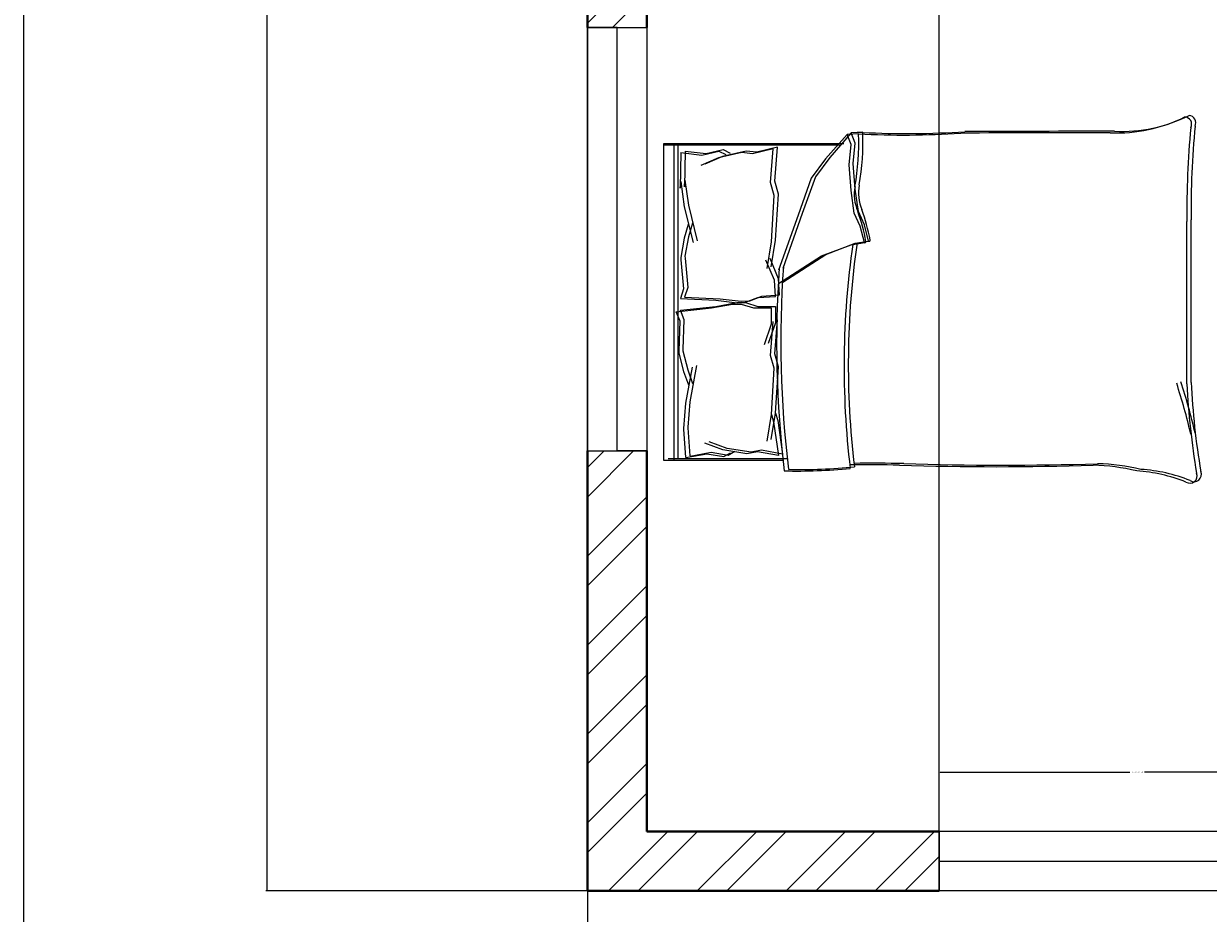
# Model space of a CAD drawing. Units: inches. Extents: x 1601 to 2297, y 1496 to 2631.
# Tile 2 of 57: x 1601 to 1780, y 1632 to 1767. Entities that reach past the tile are written whole.
import ezdxf

# ---------------------------------------------------------------- set-up
doc = ezdxf.new("R2010")
doc.units = ezdxf.units.IN
for name, color, linetype, lineweight in [('A-ANNO-DIMS', 2, 'Continuous', 18), ('A-ANNO-TTLB', 7, 'Continuous', 25), ('A-FURN', 8, 'Continuous', 18), ('A-GLAZ', 161, 'Continuous', 20), ('A-WALL', 7, 'Continuous', 40), ('A-WALL-PATT', 215, 'Continuous', 13)]:
    doc.layers.add(name, color=color, linetype=linetype, lineweight=lineweight)
doc.styles.get("Standard").update_dxf_attribs({"font": 'arial.ttf'})
doc.dimstyles.get("Standard").update_dxf_attribs({"dimtxt": 0.18, "dimasz": 0.18, "dimexe": 0.18, "dimexo": 0.0625, "dimgap": 0.09, "dimtad": 0, "dimtih": 1, "dimtoh": 1, "dimdec": 4, "dimzin": 0, "dimdsep": 46, "dimtxsty": 'Standard', "dimcen": 0.09, "dimadec": 0, "dimazin": 0, "dimtfac": 1, "dimtdec": 4, "dimtofl": 0, "dimtmove": 0, "dimatfit": 3, "dimfxl": 1, "dimtolj": 1, "dimtzin": 0, "dimarcsym": 0})

# ---------------------------------------------------------------- blocks, each defined once
blk = doc.blocks.new('BED-DOUBLE')
for p, q in [((27.75, 52.87), (24.5, 49.16)), ((27.75, 52.87), (24.5, 49.16)), ((27.75, 52.87), (24.5, 49.16)), ((27.75, 52.87), (24.5, 49.16)), ((28.39, 53.1), (25.13, 49.39)), ((28.39, 53.1), (25.13, 49.39)), ((28.39, 53.1), (25.13, 49.39)), ((28.39, 53.1), (25.13, 49.39)), ((29.49, 52.95), (27.75, 52.87, 3.87)), ((29.49, 52.95), (27.75, 52.87, 3.87)), ((29.49, 52.95), (27.75, 52.87, 3.87)), ((29.49, 52.95), (27.75, 52.87, 3.87)), ((28.36, 51.33), (27.75, 52.87)), ((28.36, 51.33), (27.75, 52.87)), ((28.36, 51.33), (27.75, 52.87)), ((28.36, 51.33), (27.75, 52.87)), ((30.13, 53.18), (28.39, 53.1, 3.87)), ((30.13, 53.18), (28.39, 53.1, 3.87)), ((30.13, 53.17), (28.39, 53.1, 3.87)), ((30.13, 53.17), (28.39, 53.1, 3.87)), ((29, 51.56), (28.39, 53.1)), ((29, 51.56), (28.39, 53.1)), ((29, 51.56), (28.39, 53.1)), ((29, 51.56), (28.39, 53.1)), ((0, 51.49), (0.64, 51.49)), ((0, 3.47), (0, 51.49)), ((0, 51.49), (0.64, 51.49)), ((0, 3.47), (0, 51.49)), ((0, 51.27), (26.61, 51.27)), ((0, 51.27), (26.61, 51.27)), ((0, 51.26), (26.61, 51.26)), ((0, 51.26), (26.61, 51.26)), ((0.64, 51.49), (27.25, 51.49)), ((0.64, 51.49), (27.25, 51.49)), ((0.64, 51.49), (27.25, 51.49)), ((0.64, 51.49), (27.25, 51.49)), ((1.53, 3.47), (1.53, 51.27)), ((1.53, 3.47), (1.53, 51.27)), ((1.53, 3.47), (1.53, 51.26)), ((1.53, 3.47), (1.53, 51.26)), ((2.17, 3.7), (2.17, 51.49)), ((2.17, 3.7), (2.17, 51.49)), ((2.17, 3.7), (2.17, 51.49)), ((2.17, 3.7), (2.17, 51.49)), ((3.2, 50.34), (3.1, 44.94)), ((3.2, 50.34), (3.1, 44.94)), ((3.2, 50.34), (3.1, 44.94)), ((3.2, 50.34), (3.1, 44.94)), ((3.2, 50.34), (6.41, 49.96)), ((3.2, 50.34), (6.41, 49.96)), ((3.2, 50.34), (6.41, 49.96)), ((3.2, 50.34), (6.41, 49.96)), ((5.77, 49.73), (8.34, 50.33)), ((5.77, 49.73), (8.34, 50.33)), ((5.77, 49.73), (8.34, 50.33)), ((5.77, 49.73), (8.34, 50.33)), ((6.41, 49.96), (8.98, 50.56)), ((6.41, 49.96), (8.98, 50.56)), ((6.41, 49.96), (8.98, 50.56)), ((6.41, 49.96), (8.98, 50.56)), ((8.34, 50.33), (9.38, 49.81)), ((8.34, 50.33), (9.38, 49.81)), ((8.34, 50.33), (9.38, 49.81)), ((8.34, 50.33), (9.38, 49.81)), ((12.47, 50.34), (8.9, 49.54)), ((12.47, 50.34), (8.9, 49.54)), ((12.47, 50.34), (8.9, 49.54)), ((12.47, 50.34), (8.9, 49.54)), ((8.98, 50.56), (10.02, 50.04)), ((8.98, 50.56), (10.02, 50.04)), ((8.98, 50.56), (10.02, 50.04)), ((8.98, 50.56), (10.02, 50.04)), ((14.07, 50.15), (12.47, 50.34)), ((14.07, 50.15), (12.47, 50.34)), ((14.07, 50.15), (12.47, 50.34)), ((14.07, 50.15), (12.47, 50.34)), ((16.57, 50.7), (13.43, 49.92)), ((16.57, 50.7), (13.43, 49.92)), ((16.57, 50.7), (13.43, 49.92)), ((16.57, 50.7), (13.43, 49.92)), ((17.21, 50.93), (14.07, 50.15)), ((17.21, 50.93), (14.07, 50.15)), ((17.21, 50.93), (14.07, 50.15)), ((17.21, 50.93), (14.07, 50.15)), ((16.17, 45.57), (16.57, 50.7)), ((16.17, 45.57), (16.57, 50.7)), ((16.17, 45.57), (16.57, 50.7)), ((16.17, 45.57), (16.57, 50.7)), ((16.81, 45.79), (17.21, 50.93)), ((16.81, 45.79), (17.21, 50.93)), ((16.81, 45.79), (17.21, 50.93)), ((16.81, 45.79), (17.21, 50.93)), ((28.06, 48.23), (28.36, 51.33)), ((28.06, 48.23), (28.36, 51.33)), ((28.06, 48.23), (28.36, 51.33)), ((28.06, 48.23), (28.36, 51.33)), ((28.69, 48.46), (29, 51.56)), ((28.69, 48.46), (29, 51.56)), ((28.69, 48.46), (29, 51.56)), ((28.69, 48.46), (29, 51.56)), ((2.56, 50.11), (2.46, 44.71)), ((2.56, 50.11), (2.46, 44.71)), ((2.56, 50.11), (2.46, 44.71)), ((2.56, 50.11), (2.46, 44.71)), ((2.56, 50.11), (5.77, 49.73)), ((2.56, 50.11), (5.77, 49.73)), ((2.56, 50.11), (5.77, 49.73)), ((2.56, 50.11), (5.77, 49.73)), ((8.26, 49.31), (5.58, 48.13)), ((8.26, 49.31), (5.58, 48.13)), ((8.26, 49.31), (5.58, 48.13)), ((8.26, 49.31), (5.58, 48.13)), ((8.9, 49.54), (6.22, 48.36)), ((8.9, 49.54), (6.22, 48.36)), ((8.9, 49.54), (6.22, 48.36)), ((8.9, 49.54), (6.22, 48.36)), ((11.83, 50.11), (8.26, 49.31)), ((11.83, 50.11), (8.26, 49.31)), ((11.83, 50.11), (8.26, 49.31)), ((11.83, 50.11), (8.26, 49.31)), ((13.43, 49.92), (11.83, 50.11)), ((13.43, 49.92), (11.83, 50.11)), ((13.43, 49.92), (11.83, 50.11)), ((13.43, 49.92), (11.83, 50.11)), ((24.5, 49.16), (22.33, 46.22)), ((24.5, 49.16), (22.33, 46.22)), ((24.5, 49.16), (22.33, 46.22)), ((24.5, 49.16), (22.33, 46.22)), ((25.13, 49.39), (22.97, 46.45)), ((25.13, 49.39), (22.97, 46.45)), ((25.13, 49.39), (22.97, 46.45)), ((25.13, 49.39), (22.97, 46.45)), ((28.36, 44.36), (28.06, 48.23)), ((28.36, 44.36), (28.06, 48.23)), ((28.36, 44.36), (28.06, 48.23)), ((28.36, 44.36), (28.06, 48.23)), ((29, 44.59), (28.69, 48.46)), ((29, 44.59), (28.69, 48.46)), ((29, 44.59), (28.69, 48.46)), ((29, 44.59), (28.69, 48.46)), ((2.46, 44.71), (2.54, 45.71)), ((2.46, 44.71), (2.54, 45.71)), ((2.46, 44.71), (2.54, 45.71)), ((2.46, 44.71), (2.54, 45.71)), ((2.54, 45.71), (3.07, 41.91)), ((2.54, 45.71), (3.07, 41.91)), ((2.54, 45.71), (3.07, 41.91)), ((2.54, 45.71), (3.07, 41.91)), ((3.1, 44.94), (3.18, 45.94)), ((3.1, 44.94), (3.18, 45.94)), ((3.1, 44.94), (3.18, 45.94)), ((3.1, 44.94), (3.18, 45.94)), ((3.18, 45.94), (3.71, 42.14)), ((3.18, 45.94), (3.71, 42.14)), ((3.18, 45.94), (3.71, 42.14)), ((3.18, 45.94), (3.71, 42.14)), ((16.73, 43.61), (16.17, 45.57)), ((16.73, 43.61), (16.17, 45.57)), ((16.73, 43.61), (16.17, 45.57)), ((16.73, 43.61), (16.17, 45.57)), ((17.37, 43.83), (16.81, 45.79)), ((17.37, 43.83), (16.81, 45.79)), ((17.37, 43.83), (16.81, 45.79)), ((17.37, 43.83), (16.81, 45.79)), ((22.33, 46.22), (20.32, 40.64)), ((22.33, 46.22), (20.32, 40.64)), ((22.33, 46.22), (20.32, 40.64)), ((22.33, 46.22), (20.32, 40.64)), ((22.97, 46.45), (20.96, 40.87)), ((22.97, 46.45), (20.96, 40.87)), ((22.97, 46.45), (20.96, 40.87)), ((22.97, 46.45), (20.96, 40.87)), ((16.3, 36.6), (16.73, 43.61)), ((16.3, 36.6), (16.73, 43.61)), ((16.3, 36.6), (16.73, 43.61)), ((16.3, 36.6), (16.73, 43.61)), ((16.93, 36.82), (17.37, 43.83)), ((16.93, 36.82), (17.37, 43.83)), ((16.93, 36.82), (17.37, 43.83)), ((16.93, 36.82), (17.37, 43.83)), ((28.83, 40.95), (28.36, 44.36)), ((28.83, 40.95), (28.36, 44.36)), ((28.83, 40.95), (28.36, 44.36)), ((28.83, 40.95), (28.36, 44.36)), ((29.47, 41.18), (29, 44.59)), ((29.47, 41.18), (29, 44.59)), ((29.47, 41.18), (29, 44.59)), ((29.47, 41.18), (29, 44.59)), ((3.07, 41.91), (4.42, 36.49)), ((3.07, 41.91), (4.42, 36.49)), ((3.07, 41.91), (4.42, 36.49)), ((3.07, 41.91), (4.42, 36.49)), ((3.71, 42.14), (5.06, 36.72)), ((3.71, 42.14), (5.06, 36.72)), ((3.71, 42.14), (5.06, 36.72)), ((3.71, 42.14), (5.06, 36.72)), ((20.32, 40.64), (17.38, 32.31)), ((20.32, 40.64), (17.38, 32.31)), ((20.32, 40.64), (17.38, 32.31)), ((20.32, 40.64), (17.38, 32.31)), ((20.96, 40.87), (18.02, 32.53)), ((20.96, 40.87), (18.02, 32.53)), ((20.96, 40.87), (18.02, 32.53)), ((20.96, 40.87), (18.02, 32.53)), ((29.76, 38.94), (28.83, 40.95)), ((29.76, 38.94), (28.83, 40.95)), ((29.76, 38.94), (28.83, 40.95)), ((29.76, 38.94), (28.83, 40.95)), ((30.4, 39.17), (29.47, 41.18)), ((30.4, 39.17), (29.47, 41.18)), ((30.4, 39.17), (29.47, 41.18)), ((30.4, 39.17), (29.47, 41.18)), ((79.24, 15.06), (79.24, 39.68)), ((79.24, 15.06), (79.24, 39.68)), ((79.24, 15.06), (79.24, 39.68)), ((79.24, 15.06), (79.24, 39.68)), ((79.88, 15.29), (79.88, 39.91)), ((79.88, 15.29), (79.88, 39.91)), ((79.88, 15.29), (79.88, 39.91)), ((79.88, 15.29), (79.88, 39.91)), ((3.67, 39.2), (3.08, 37.14)), ((3.67, 39.2), (3.08, 37.13)), ((3.67, 39.2), (3.08, 37.14)), ((3.67, 39.2), (3.08, 37.13)), ((4.31, 39.43), (3.72, 37.36)), ((4.31, 39.43), (3.72, 37.36)), ((4.31, 39.43), (3.72, 37.36)), ((4.31, 39.43), (3.72, 37.36)), ((30.38, 36.46), (29.76, 38.94)), ((30.38, 36.46), (29.76, 38.94)), ((30.38, 36.46), (29.76, 38.94)), ((30.38, 36.46), (29.76, 38.94)), ((31.02, 36.69), (30.4, 39.17)), ((31.02, 36.69), (30.4, 39.17)), ((31.02, 36.69), (30.4, 39.17)), ((31.02, 36.69), (30.4, 39.17)), ((3.08, 37.14), (2.54, 34.2)), ((3.08, 37.14), (2.54, 34.2)), ((3.08, 37.13), (2.54, 34.2)), ((3.08, 37.13), (2.54, 34.2)), ((3.72, 37.36), (3.18, 34.43)), ((3.72, 37.36), (3.18, 34.43)), ((3.72, 37.36), (3.18, 34.43)), ((3.72, 37.36), (3.18, 34.43)), ((15.63, 32.56), (16.3, 36.6)), ((15.63, 32.56), (16.3, 36.6)), ((15.63, 32.56), (16.3, 36.6)), ((15.63, 32.56), (16.3, 36.6)), ((16.27, 32.79), (16.93, 36.82)), ((16.27, 32.79), (16.93, 36.82)), ((16.27, 32.79), (16.93, 36.82)), ((16.27, 32.79), (16.93, 36.82)), ((23.88, 34.45), (28.36, 36.15)), ((23.88, 34.45), (28.36, 36.15)), ((23.88, 34.45), (28.36, 36.15)), ((23.88, 34.45), (28.36, 36.15)), ((24.52, 34.68), (29, 36.38)), ((24.52, 34.68), (29, 36.38)), ((24.52, 34.68), (29, 36.38)), ((24.52, 34.68), (29, 36.38)), ((28.36, 36.15), (30.38, 36.46)), ((28.36, 36.15), (30.38, 36.46)), ((28.36, 36.15), (30.38, 36.46)), ((28.36, 36.15), (30.38, 36.46)), ((29, 36.38), (31.02, 36.69)), ((29, 36.38), (31.02, 36.69)), ((29, 36.38), (31.02, 36.69)), ((29, 36.38), (31.02, 36.69)), ((2.54, 34.2), (2.56, 33.88)), ((2.54, 34.2), (2.56, 33.88)), ((2.54, 34.2), (2.56, 33.88)), ((2.54, 34.2), (2.56, 33.88)), ((3.18, 34.43), (3.2, 34.11)), ((3.18, 34.43), (3.2, 34.11)), ((3.18, 34.43), (3.2, 34.11)), ((3.18, 34.43), (3.2, 34.11)), ((3.2, 34.11), (3.62, 29.68)), ((3.2, 34.11), (3.62, 29.68)), ((3.2, 34.11), (3.62, 29.68)), ((3.2, 34.11), (3.62, 29.68)), ((17.38, 30.26), (23.88, 34.45)), ((17.38, 30.26), (23.88, 34.45)), ((17.38, 30.26), (23.88, 34.45)), ((17.38, 30.26), (23.88, 34.45)), ((18.02, 30.49), (24.52, 34.68)), ((18.02, 30.49), (24.52, 34.68)), ((18.02, 30.49), (24.52, 34.68)), ((18.02, 30.49), (24.52, 34.68)), ((2.56, 33.88), (2.98, 29.46)), ((2.56, 33.88), (2.98, 29.46)), ((2.56, 33.88), (2.98, 29.46)), ((2.56, 33.88), (2.98, 29.46)), ((16.74, 30.75), (15.45, 33.82)), ((16.74, 30.75), (15.45, 33.82)), ((16.74, 30.75), (15.45, 33.82)), ((16.74, 30.75), (15.45, 33.82)), ((17.38, 30.98), (16.09, 34.05)), ((17.38, 30.98), (16.09, 34.05)), ((17.38, 30.98), (16.09, 34.05)), ((17.38, 30.98), (16.09, 34.05)), ((16.89, 28.3), (16.74, 30.75)), ((16.89, 28.3), (16.74, 30.75)), ((16.89, 28.3), (16.74, 30.75)), ((16.89, 28.3), (16.74, 30.75)), ((17.53, 28.53), (17.38, 30.98)), ((17.53, 28.53), (17.38, 30.98)), ((17.53, 28.53), (17.38, 30.98)), ((17.53, 28.53), (17.38, 30.98)), ((2.98, 29.46), (2.49, 27.98)), ((2.98, 29.46), (2.49, 27.98)), ((2.98, 29.46), (2.49, 27.98)), ((2.98, 29.46), (2.49, 27.98)), ((3.62, 29.68), (3.13, 28.21)), ((3.62, 29.68), (3.13, 28.2)), ((3.62, 29.68), (3.13, 28.21)), ((3.62, 29.68), (3.13, 28.2)), ((2.49, 27.98), (7.87, 27.73)), ((2.49, 27.98), (7.87, 27.73)), ((2.49, 27.98), (7.87, 27.73)), ((2.49, 27.98), (7.87, 27.73)), ((3.13, 28.21), (8.51, 27.96)), ((3.13, 28.21), (8.51, 27.96)), ((3.13, 28.2), (8.51, 27.96)), ((3.13, 28.2), (8.51, 27.96)), ((7.22, 26.56), (10.4, 27.14)), ((7.22, 26.56), (10.4, 27.14)), ((7.22, 26.56), (10.4, 27.14)), ((7.22, 26.56), (10.4, 27.14)), ((7.86, 26.79), (11.04, 27.37)), ((7.86, 26.79), (11.04, 27.37)), ((7.86, 26.79), (11.04, 27.37)), ((7.86, 26.79), (11.04, 27.37)), ((7.87, 27.73), (11.08, 27.35)), ((7.87, 27.73), (11.08, 27.35)), ((7.87, 27.73), (11.08, 27.35)), ((7.87, 27.73), (11.08, 27.35)), ((8.51, 27.96), (11.72, 27.58)), ((8.51, 27.96), (11.72, 27.58)), ((8.51, 27.96), (11.72, 27.58)), ((8.51, 27.96), (11.72, 27.58)), ((10.4, 27.14), (11.7, 27.14)), ((10.4, 27.14), (11.7, 27.14)), ((10.4, 27.14), (11.7, 27.14)), ((10.4, 27.14), (11.7, 27.14)), ((11.04, 27.37), (12.34, 27.37)), ((11.04, 27.37), (12.34, 27.37)), ((11.04, 27.37), (12.34, 27.37)), ((11.04, 27.37), (12.34, 27.37)), ((11.08, 27.35), (12.38, 27.44)), ((11.08, 27.35), (12.38, 27.44)), ((11.08, 27.35), (12.38, 27.44)), ((11.08, 27.35), (12.38, 27.44)), ((11.7, 27.14), (13.58, 26.56)), ((11.7, 27.14), (13.58, 26.56)), ((11.7, 27.14), (13.58, 26.56)), ((11.7, 27.14), (13.58, 26.56)), ((11.72, 27.58), (13.02, 27.66)), ((11.72, 27.58), (13.02, 27.66)), ((11.72, 27.58), (13.02, 27.66)), ((11.72, 27.58), (13.02, 27.66)), ((12.34, 27.37), (14.22, 26.79)), ((12.34, 27.37), (14.22, 26.79)), ((12.34, 27.37), (14.22, 26.79)), ((12.34, 27.37), (14.22, 26.79)), ((12.38, 27.44), (14.22, 28.13)), ((12.38, 27.44), (14.22, 28.13)), ((12.38, 27.44), (14.22, 28.13)), ((12.38, 27.44), (14.22, 28.13)), ((13.02, 27.66), (14.86, 28.36)), ((13.02, 27.66), (14.86, 28.36)), ((13.02, 27.66), (14.86, 28.36)), ((13.02, 27.66), (14.86, 28.36)), ((14.22, 28.13), (16.89, 28.3)), ((14.22, 28.13), (16.89, 28.3)), ((14.22, 28.13), (16.89, 28.3)), ((14.22, 28.13), (16.89, 28.3)), ((14.86, 28.36), (17.53, 28.53)), ((14.86, 28.36), (17.53, 28.53)), ((14.86, 28.36), (17.53, 28.53)), ((14.86, 28.36), (17.53, 28.53)), ((1.87, 25.98), (7.22, 26.56)), ((1.87, 25.98), (7.22, 26.56)), ((1.87, 25.98), (7.22, 26.56)), ((1.87, 25.98), (7.22, 26.56)), ((2.45, 24.54), (1.87, 25.98)), ((2.45, 24.54), (1.87, 25.98)), ((2.45, 24.54), (1.87, 25.98)), ((2.45, 24.54), (1.87, 25.98)), ((2.51, 26.21), (7.86, 26.79)), ((2.51, 26.21), (7.86, 26.79)), ((2.51, 26.21), (7.86, 26.79)), ((2.51, 26.21), (7.86, 26.79)), ((3.09, 24.77), (2.51, 26.21)), ((3.09, 24.76), (2.51, 26.21)), ((3.09, 24.77), (2.51, 26.21)), ((3.09, 24.76), (2.51, 26.21)), ((13.58, 26.56), (16.26, 26.56)), ((13.58, 26.56), (16.26, 26.56)), ((13.58, 26.56), (16.26, 26.56)), ((13.58, 26.56), (16.26, 26.56)), ((14.22, 26.79), (16.9, 26.79)), ((14.22, 26.79), (16.9, 26.79)), ((14.22, 26.79), (16.9, 26.79)), ((14.22, 26.79), (16.9, 26.79)), ((16.26, 26.56), (16.26, 24.1)), ((16.26, 26.56), (16.26, 24.1)), ((16.26, 26.56), (16.26, 24.1)), ((16.26, 26.56), (16.26, 24.1)), ((16.9, 26.79), (16.9, 24.33)), ((16.9, 26.79), (16.9, 24.33)), ((16.9, 26.79), (16.9, 24.33)), ((16.9, 26.79), (16.9, 24.33)), ((2.3, 20.09), (2.45, 24.54)), ((2.3, 20.09), (2.45, 24.54)), ((2.3, 20.09), (2.45, 24.54)), ((2.3, 20.09), (2.45, 24.54)), ((2.94, 20.32), (3.09, 24.77)), ((2.94, 20.32), (3.09, 24.77)), ((2.94, 20.32), (3.09, 24.76)), ((2.94, 20.32), (3.09, 24.76)), ((16.26, 24.1), (15.17, 20.96)), ((16.26, 24.1), (15.17, 20.96)), ((16.26, 24.1), (15.17, 20.96)), ((16.26, 24.1), (15.17, 20.96)), ((16.9, 24.33), (15.81, 21.19)), ((16.9, 24.33), (15.81, 21.19)), ((16.9, 24.33), (15.81, 21.19)), ((16.9, 24.33), (15.81, 21.19)), ((16.17, 19.38), (16.57, 24.52)), ((16.17, 19.38), (16.57, 24.52)), ((16.17, 19.38), (16.57, 24.52)), ((16.17, 19.38), (16.57, 24.52)), ((16.81, 19.61), (17.21, 24.74)), ((16.81, 19.61), (17.21, 24.74)), ((16.81, 19.61), (17.21, 24.74)), ((16.81, 19.61), (17.21, 24.74)), ((2.3, 19.77), (2.3, 20.09)), ((2.3, 19.77), (2.3, 20.09)), ((2.3, 19.77), (2.3, 20.09)), ((2.3, 19.77), (2.3, 20.09)), ((3.03, 16.88), (2.3, 19.77)), ((3.03, 16.88), (2.3, 19.77)), ((3.03, 16.88), (2.3, 19.77)), ((3.03, 16.88), (2.3, 19.77)), ((2.94, 20), (2.94, 20.32)), ((2.94, 20), (2.94, 20.32)), ((2.94, 20), (2.94, 20.32)), ((2.94, 20), (2.94, 20.32)), ((3.67, 17.11), (2.94, 20)), ((3.67, 17.11), (2.94, 20)), ((3.67, 17.11), (2.94, 20)), ((3.67, 17.11), (2.94, 20)), ((16.73, 17.42), (16.17, 19.38)), ((16.73, 17.42), (16.17, 19.38)), ((16.73, 17.42), (16.17, 19.38)), ((16.73, 17.42), (16.17, 19.38)), ((17.37, 17.65), (16.81, 19.61)), ((17.37, 17.65), (16.81, 19.61)), ((17.37, 17.65), (16.81, 19.61)), ((17.37, 17.65), (16.81, 19.61)), ((3.75, 14.85), (3.03, 16.88)), ((3.75, 14.85), (3.03, 16.88)), ((3.75, 14.85), (3.03, 16.88)), ((3.75, 14.85), (3.03, 16.88)), ((3.32, 12.11), (4.33, 17.6)), ((3.32, 12.11), (4.33, 17.6)), ((3.32, 12.11), (4.33, 17.6)), ((3.32, 12.11), (4.33, 17.6)), ((4.39, 15.08), (3.67, 17.11)), ((4.39, 15.08), (3.67, 17.11)), ((4.39, 15.08), (3.67, 17.11)), ((4.39, 15.08), (3.67, 17.11)), ((3.96, 12.34), (4.97, 17.83)), ((3.96, 12.34), (4.97, 17.83)), ((3.96, 12.34), (4.97, 17.83)), ((3.96, 12.34), (4.97, 17.83)), ((16.3, 10.41), (16.73, 17.42)), ((16.3, 10.41), (16.73, 17.42)), ((16.3, 10.41), (16.73, 17.42)), ((16.3, 10.41), (16.73, 17.42)), ((16.93, 10.64), (17.37, 17.65)), ((16.93, 10.64), (17.37, 17.65)), ((16.93, 10.64), (17.37, 17.65)), ((16.93, 10.64), (17.37, 17.65)), ((3.03, 8.28), (3.32, 12.11)), ((3.03, 8.28), (3.32, 12.11)), ((3.03, 8.28), (3.32, 12.11)), ((3.03, 8.28), (3.32, 12.11)), ((3.67, 8.51), (3.96, 12.34)), ((3.67, 8.51), (3.96, 12.34)), ((3.67, 8.51), (3.96, 12.34)), ((3.67, 8.51), (3.96, 12.34)), ((15.63, 6.38), (16.3, 10.41)), ((15.63, 6.38), (16.3, 10.41)), ((15.63, 6.38), (16.3, 10.41)), ((15.63, 6.38), (16.3, 10.41)), ((16.27, 6.61), (16.93, 10.64)), ((16.27, 6.61), (16.93, 10.64)), ((16.27, 6.61), (16.93, 10.64)), ((16.27, 6.61), (16.93, 10.64)), ((16.3, 10.41), (16.62, 9.28)), ((16.3, 10.41), (16.62, 9.28)), ((16.3, 10.41), (16.62, 9.28)), ((16.3, 10.41), (16.62, 9.28)), ((16.62, 9.28), (17.34, 4.18)), ((16.62, 9.28), (17.34, 4.18)), ((16.62, 9.28), (17.34, 4.18)), ((16.62, 9.28), (17.34, 4.18)), ((16.93, 10.64), (17.26, 9.51)), ((16.93, 10.64), (17.26, 9.51)), ((16.93, 10.64), (17.26, 9.51)), ((16.93, 10.64), (17.26, 9.51)), ((17.26, 9.51), (17.98, 4.41)), ((17.26, 9.51), (17.98, 4.41)), ((17.26, 9.51), (17.98, 4.41)), ((17.26, 9.51), (17.98, 4.41)), ((3.01, 8.18), (3.03, 8.28)), ((3.01, 8.18), (3.03, 8.28)), ((3.01, 8.18), (3.03, 8.28)), ((3.01, 8.18), (3.03, 8.28)), ((3.34, 3.9), (3.01, 8.18)), ((3.34, 3.9), (3.01, 8.18)), ((3.34, 3.9), (3.01, 8.18)), ((3.34, 3.9), (3.01, 8.18)), ((3.65, 8.41), (3.67, 8.51)), ((3.65, 8.41), (3.67, 8.51)), ((3.65, 8.41), (3.67, 8.51)), ((3.65, 8.41), (3.67, 8.51)), ((3.98, 4.13), (3.65, 8.41)), ((3.98, 4.13), (3.65, 8.41)), ((3.98, 4.13), (3.65, 8.41)), ((3.98, 4.13), (3.65, 8.41)), ((8.95, 5.05), (6.21, 6.06)), ((8.95, 5.05), (6.21, 6.06)), ((8.95, 5.05), (6.21, 6.06)), ((8.95, 5.05), (6.21, 6.06)), ((9.59, 5.28), (6.85, 6.29)), ((9.59, 5.28), (6.85, 6.29)), ((9.59, 5.28), (6.85, 6.29)), ((9.59, 5.28), (6.85, 6.29)), ((18.75, 3.7), (0.64, 3.7)), ((18.75, 3.7), (0.64, 3.7)), ((18.75, 3.7), (0.64, 3.7)), ((18.75, 3.7), (0.64, 3.7)), ((3.32, 3.89), (6.5, 4.47)), ((3.32, 3.89), (6.5, 4.47)), ((3.32, 3.89), (6.5, 4.47)), ((3.32, 3.89), (6.5, 4.47)), ((3.96, 4.12), (7.14, 4.7)), ((3.96, 4.12), (7.14, 4.7)), ((3.96, 4.12), (7.14, 4.7)), ((3.96, 4.12), (7.14, 4.7)), ((6.5, 4.47), (9.1, 4.04)), ((6.5, 4.47), (9.1, 4.04)), ((6.5, 4.47), (9.1, 4.04)), ((6.5, 4.47), (9.1, 4.04)), ((7.14, 4.7), (9.74, 4.27)), ((7.14, 4.7), (9.74, 4.27)), ((7.14, 4.7), (9.74, 4.27)), ((7.14, 4.7), (9.74, 4.27)), ((12.57, 4.47), (8.95, 5.05)), ((12.57, 4.47), (8.95, 5.05)), ((12.57, 4.47), (8.95, 5.05)), ((12.57, 4.47), (8.95, 5.05)), ((9.1, 4.04), (10.11, 4.62)), ((9.1, 4.04), (10.11, 4.62)), ((9.1, 4.04), (10.11, 4.62)), ((9.1, 4.04), (10.11, 4.62)), ((13.21, 4.7), (9.59, 5.28)), ((13.21, 4.7), (9.59, 5.28)), ((13.21, 4.7), (9.59, 5.28)), ((13.21, 4.7), (9.59, 5.28)), ((9.74, 4.27), (10.75, 4.85)), ((9.74, 4.27), (10.75, 4.85)), ((9.74, 4.27), (10.75, 4.85)), ((9.74, 4.27), (10.75, 4.85)), ((14.16, 4.76), (12.57, 4.47)), ((14.16, 4.76), (12.57, 4.47)), ((14.16, 4.76), (12.57, 4.47)), ((14.16, 4.76), (12.57, 4.47)), ((14.8, 4.99), (13.21, 4.7)), ((14.8, 4.99), (13.21, 4.7)), ((14.8, 4.99), (13.21, 4.7)), ((14.8, 4.99), (13.21, 4.7)), ((17.34, 4.18), (14.16, 4.76)), ((17.34, 4.18), (14.16, 4.76)), ((17.34, 4.18), (14.16, 4.76)), ((17.34, 4.18), (14.16, 4.76)), ((17.98, 4.41), (14.8, 4.99)), ((17.98, 4.41), (14.8, 4.99)), ((17.98, 4.41), (14.8, 4.99)), ((17.98, 4.41), (14.8, 4.99)), ((18.11, 3.47), (0, 3.47)), ((18.11, 3.47), (0, 3.47)), ((18.11, 3.47), (0, 3.47)), ((18.11, 3.47), (0, 3.47))]:
    blk.add_line(p, q)
for centre, radius, start, end in [((69.31, 76.39), 23.07, 267.4714, 296.4681), ((69.31, 76.39), 23.07, 267.4714, 296.4681), ((69.31, 76.39), 23.07, 267.4714, 296.4681), ((69.31, 76.39), 23.07, 267.4714, 296.4681), ((79.51, 54.64), 1.1, 332.6588, 86.02), ((79.51, 54.64), 1.1, 332.6588, 86.02), ((79.51, 54.64), 1.1, 332.6588, 86.02), ((79.51, 54.64), 1.1, 332.6588, 86.02), ((68.67, 76.16), 23.07, 267.4714, 296.4681), ((68.67, 76.16), 23.07, 267.4714, 296.4681), ((68.67, 76.16), 23.07, 267.4714, 296.4681), ((68.67, 76.16), 23.07, 267.4714, 296.4681), ((78.87, 54.41), 1.1, 332.6588, 86.02), ((78.87, 54.41), 1.1, 332.6588, 86.02), ((78.87, 54.41), 1.1, 332.6588, 86.02), ((78.87, 54.41), 1.1, 332.6588, 86.02), ((212.28, 41.15), 133.04, 174.4998, 180.6351), ((212.28, 41.15), 133.04, 174.4998, 180.6351), ((212.28, 41.15), 133.04, 174.4998, 180.6351), ((212.28, 41.15), 133.04, 174.4998, 180.6351), ((212.92, 41.38), 133.04, 174.4998, 180.6351), ((212.92, 41.38), 133.04, 174.4998, 180.6351), ((212.92, 41.38), 133.04, 174.4998, 180.6351), ((212.92, 41.38), 133.04, 174.4998, 180.6351), ((-6.66, 51.33), 36.18, 349.8763, 2.5657), ((-6.66, 51.33), 36.18, 349.8763, 2.5657), ((-6.66, 51.33), 36.18, 349.8763, 2.5657), ((-6.66, 51.33), 36.18, 349.8763, 2.5657), ((36.31, 182.27), 129.5, 266.9791, 273.8365), ((36.31, 182.27), 129.5, 266.9791, 273.8365), ((36.31, 182.27), 129.5, 266.9791, 273.8365), ((36.31, 182.27), 129.5, 266.9791, 273.8365), ((-6.02, 51.56), 36.18, 349.8763, 2.5657), ((-6.02, 51.56), 36.18, 349.8763, 2.5657), ((-6.02, 51.56), 36.18, 349.8763, 2.5657), ((-6.02, 51.56), 36.18, 349.8763, 2.5657), ((36.95, 182.49), 129.5, 266.9791, 273.8365), ((36.95, 182.49), 129.5, 266.9791, 273.8365), ((36.95, 182.49), 129.5, 266.9791, 273.8365), ((36.95, 182.49), 129.5, 266.9791, 273.8365), ((67.82, -4508.74), 4561.86, 90.00217, 90.28689), ((67.82, -4508.74), 4561.86, 90.00217, 90.28689), ((67.82, -4508.74), 4561.86, 90.00217, 90.28689), ((67.82, -4508.74), 4561.86, 90.00217, 90.28689), ((68.46, -4508.52), 4561.86, 90.00217, 90.28689), ((68.46, -4508.52), 4561.86, 90.00217, 90.28689), ((68.46, -4508.52), 4561.86, 90.00217, 90.28689), ((68.46, -4508.52), 4561.86, 90.00217, 90.28689), ((35.07, 43.74), 6.22, 168.6608, 203.7384), ((35.07, 43.74), 6.22, 168.6608, 203.7384), ((35.07, 43.74), 6.22, 168.6608, 203.7384), ((35.07, 43.74), 6.22, 168.6608, 203.7384), ((35.71, 43.97), 6.22, 168.6608, 203.7384), ((35.71, 43.97), 6.22, 168.6608, 203.7384), ((35.71, 43.97), 6.22, 168.6608, 203.7384), ((35.71, 43.97), 6.22, 168.6608, 203.7384), ((2.12, 31.38), 29.65, 10.6617, 19.8806), ((2.12, 31.38), 29.65, 10.6617, 19.8806), ((2.12, 31.38), 29.65, 10.6617, 19.8806), ((2.12, 31.38), 29.65, 10.6617, 19.8806), ((1.48, 31.15), 29.65, 10.6617, 19.8806), ((1.48, 31.15), 29.65, 10.6617, 19.8806), ((1.48, 31.15), 29.65, 10.6617, 19.8806), ((1.48, 31.15), 29.65, 10.6617, 19.8806), ((156.32, 17.76), 129.02, 171.7845, 186.9006), ((156.32, 17.76), 129.02, 171.7845, 186.9006), ((156.32, 17.76), 129.02, 171.7845, 186.9006), ((156.32, 17.76), 129.02, 171.7845, 186.9006), ((156.96, 17.98), 129.02, 171.7845, 186.9006), ((156.96, 17.98), 129.02, 171.7845, 186.9006), ((156.96, 17.98), 129.02, 171.7845, 186.9006), ((156.96, 17.98), 129.02, 171.7845, 186.9006), ((30.44, 36.64), 0.185, 250.2464, 1.1377), ((30.44, 36.64), 0.185, 250.2464, 1.1377), ((30.44, 36.64), 0.185, 250.2464, 1.1377), ((30.44, 36.64), 0.185, 250.2464, 1.1377), ((31.08, 36.86), 0.185, 250.2464, 1.1377), ((31.08, 36.86), 0.185, 250.2464, 1.1377), ((31.08, 36.86), 0.185, 250.2464, 1.1377), ((31.08, 36.86), 0.185, 250.2464, 1.1377), ((182.05, 21.36), 164.97, 176.0865, 186.7821), ((182.05, 21.36), 164.97, 176.0865, 186.7821), ((182.05, 21.36), 164.97, 176.0865, 186.7821), ((182.05, 21.36), 164.97, 176.0865, 186.7821), ((182.69, 21.59), 164.97, 176.0865, 186.7821), ((182.69, 21.59), 164.97, 176.0865, 186.7821), ((182.69, 21.59), 164.97, 176.0865, 186.7821), ((182.69, 21.59), 164.97, 176.0865, 186.7821), ((-23.71, -17.22), 106.46, 13.3832, 17.7053), ((-23.71, -17.22), 106.46, 13.3832, 17.7053), ((-23.71, -17.22), 106.46, 13.3832, 17.7053), ((-23.71, -17.22), 106.46, 13.3832, 17.7053), ((-23.07, -16.99), 106.46, 13.3832, 17.7053), ((-23.07, -16.99), 106.46, 13.3832, 17.7053), ((-23.07, -16.99), 106.46, 13.3832, 17.7053), ((-23.07, -16.99), 106.46, 13.3832, 17.7053), ((200.84, 21.43), 121.76, 182.9958, 189.4091), ((200.84, 21.43), 121.76, 182.9958, 189.4091), ((200.84, 21.43), 121.76, 182.9958, 189.4091), ((200.84, 21.43), 121.76, 182.9958, 189.4091), ((201.48, 21.65), 121.76, 182.9958, 189.4091), ((201.48, 21.65), 121.76, 182.9958, 189.4091), ((201.48, 21.65), 121.76, 182.9958, 189.4091), ((201.48, 21.65), 121.76, 182.9958, 189.4091), ((20.1, 85.16), 83.31, 268.7218, 275.604), ((20.1, 85.16), 83.31, 268.7218, 275.604), ((20.1, 85.16), 83.31, 268.7218, 275.604), ((20.1, 85.16), 83.31, 268.7218, 275.604), ((20.74, 85.39), 83.31, 268.7218, 275.604), ((20.74, 85.39), 83.31, 268.7218, 275.604), ((20.74, 85.39), 83.31, 268.7218, 275.604), ((20.74, 85.39), 83.31, 268.7218, 275.604), ((31.17, -167.31), 170.11, 88.4762, 91.0082), ((31.17, -167.31), 170.11, 88.4762, 91.0082), ((31.17, -167.31), 170.11, 88.4762, 91.0082), ((31.17, -167.31), 170.11, 88.4762, 91.0082), ((31.81, -167.08), 170.11, 88.4762, 91.0082), ((31.81, -167.08), 170.11, 88.4762, 91.0082), ((31.81, -167.08), 170.11, 88.4762, 91.0082), ((31.81, -167.08), 170.11, 88.4762, 91.0082), ((50.61, 484.82), 482.31, 268.2277, 271.7185), ((50.61, 484.82), 482.31, 268.2277, 271.7185), ((50.61, 484.82), 482.31, 268.2277, 271.7185), ((50.61, 484.82), 482.31, 268.2277, 271.7185), ((51.25, 485.05), 482.31, 268.2277, 271.7185), ((51.25, 485.05), 482.31, 268.2277, 271.7185), ((51.25, 485.05), 482.31, 268.2277, 271.7185), ((51.25, 485.05), 482.31, 268.2277, 271.7185), ((64.51, -26.9), 29.63, 76.0648, 88.9113), ((64.51, -26.9), 29.63, 76.0648, 88.9113), ((64.51, -26.9), 29.63, 76.0648, 88.9113), ((64.51, -26.9), 29.63, 76.0648, 88.9113), ((65.15, -26.67), 29.63, 76.0648, 88.9113), ((65.15, -26.67), 29.63, 76.0648, 88.9113), ((65.15, -26.67), 29.63, 76.0648, 88.9113), ((65.15, -26.67), 29.63, 76.0648, 88.9113), ((70.28, -21.66), 23.56, 67.9751, 86.652), ((70.28, -21.66), 23.56, 67.9751, 86.652), ((70.28, -21.66), 23.56, 67.9751, 86.652), ((70.28, -21.66), 23.56, 67.9751, 86.652), ((70.91, -21.43), 23.56, 67.9751, 86.652), ((70.91, -21.43), 23.56, 67.9751, 86.652), ((70.91, -21.43), 23.56, 67.9751, 86.652), ((70.91, -21.43), 23.56, 67.9751, 86.652), ((79.72, 1.09), 1.09, 236.1736, 23.4781), ((79.72, 1.09), 1.09, 236.1736, 23.4781), ((79.72, 1.09), 1.09, 236.1736, 23.4781), ((79.72, 1.09), 1.09, 236.1736, 23.4781), ((80.36, 1.32), 1.09, 236.1736, 23.4781), ((80.36, 1.32), 1.09, 236.1736, 23.4781), ((80.36, 1.32), 1.09, 236.1736, 23.4781), ((80.36, 1.32), 1.09, 236.1736, 23.4781)]:
    blk.add_arc(centre, radius, start, end)
blk = doc.blocks.new('WIN-60IN-JAMB9')
for p, q in [((4.5, 60), (0, 60)), ((0, 60), (9, 60)), ((0, 60), (0, 0)), ((4.5, 0), (4.5, 60)), ((9, 60), (9, 0)), ((0, 0), (9, 0)), ((9, 0), (4.5, 0))]:
    blk.add_line(p, q)
blk = doc.blocks.new('*D14')
at = {"layer": 'A-ANNO-DIMS', "color": 0, "lineweight": -2, "transparency": 16777216}
for p, q in [((1739.33, 1644.39), (1739.33, 1653.51)), ((1799.33, 1644.39), (1799.33, 1653.51)), ((1739.51, 1653.33), (1768.22, 1653.33)), ((1799.15, 1653.33), (1770.45, 1653.33))]:
    blk.add_line(p, q, dxfattribs=at)
at = {"layer": 'A-ANNO-DIMS', "color": 0, "transparency": 16777216}
for points in [[(1739.51, 1653.36), (1739.51, 1653.3), (1739.33, 1653.33)], [(1799.15, 1653.36), (1799.15, 1653.3), (1799.33, 1653.33)]]:
    blk.add_solid(points, dxfattribs=at)
at = {"layer": 'Defpoints', "color": 0, "transparency": 16777216}
for p in [(1799.33, 1653.33), (1739.33, 1644.33), (1799.33, 1644.33)]:
    blk.add_point(p, dxfattribs=at)
at = {"layer": 'A-ANNO-DIMS', "color": 0, "transparency": 16777216, "insert": (1769.33, 1653.33), "char_height": 0.18, "attachment_point": 5}
blk.add_mtext('\\A1;WINDOW 60 TYP.', dxfattribs=at)
blk = doc.blocks.new('*D30')
at = {"layer": 'A-ANNO-DIMS', "color": 0, "lineweight": -2, "transparency": 16777216}
for p, q in [((1685.97, 2031.33), (1637.31, 2031.33)), ((1637.49, 2031.15), (1637.49, 1833.51)), ((1637.49, 1635.51), (1637.49, 1833.14)), ((1685.97, 1635.33), (1637.31, 1635.33))]:
    blk.add_line(p, q, dxfattribs=at)
at = {"layer": 'A-ANNO-DIMS', "color": 0, "transparency": 16777216}
for points in [[(1637.46, 2031.15), (1637.52, 2031.15), (1637.49, 2031.33)], [(1637.46, 1635.51), (1637.52, 1635.51), (1637.49, 1635.33)]]:
    blk.add_solid(points, dxfattribs=at)
at = {"layer": 'Defpoints', "color": 0, "transparency": 16777216}
for p in [(1637.49, 2031.33), (1686.04, 2031.33), (1686.04, 1635.33)]:
    blk.add_point(p, dxfattribs=at)
at = {"layer": 'A-ANNO-DIMS', "color": 0, "transparency": 16777216, "insert": (1637.49, 1833.33), "char_height": 0.18, "attachment_point": 5}
blk.add_mtext('\\A1;396', dxfattribs=at)
blk = doc.blocks.new('*D34')
at = {"layer": 'A-ANNO-DIMS', "color": 0, "lineweight": -2, "transparency": 16777216}
for p, q in [((1686.04, 1635.26), (1686.04, 1513.75)), ((1893.04, 1635.26), (1893.04, 1513.75)), ((1686.22, 1513.93), (1789.25, 1513.93)), ((1892.86, 1513.93), (1789.83, 1513.93))]:
    blk.add_line(p, q, dxfattribs=at)
at = {"layer": 'A-ANNO-DIMS', "color": 0, "transparency": 16777216}
for points in [[(1686.22, 1513.96), (1686.22, 1513.9), (1686.04, 1513.93)], [(1892.86, 1513.96), (1892.86, 1513.9), (1893.04, 1513.93)]]:
    blk.add_solid(points, dxfattribs=at)
at = {"layer": 'Defpoints', "color": 0, "transparency": 16777216}
for p in [(1686.04, 1635.33), (1893.04, 1635.33), (1893.04, 1513.93)]:
    blk.add_point(p, dxfattribs=at)
at = {"layer": 'A-ANNO-DIMS', "color": 0, "transparency": 16777216, "insert": (1789.54, 1513.93), "char_height": 0.18, "attachment_point": 5}
blk.add_mtext('\\A1;207', dxfattribs=at)
blk = doc.blocks.new('*D36')
at = {"layer": 'A-ANNO-DIMS', "color": 0, "lineweight": -2, "transparency": 16777216}
for p, q in [((1686.04, 1635.39), (1686.04, 2581.06)), ((1686.22, 2580.88), (1712.36, 2580.88)), ((1739.15, 2580.88), (1713.01, 2580.88)), ((1739.33, 1635.39), (1739.33, 2581.06))]:
    blk.add_line(p, q, dxfattribs=at)
at = {"layer": 'A-ANNO-DIMS', "color": 0, "transparency": 16777216}
for points in [[(1686.22, 2580.91), (1686.22, 2580.85), (1686.04, 2580.88)], [(1739.15, 2580.91), (1739.15, 2580.85), (1739.33, 2580.88)]]:
    blk.add_solid(points, dxfattribs=at)
at = {"layer": 'Defpoints', "color": 0, "transparency": 16777216}
for p in [(1739.33, 2580.88), (1686.04, 1635.33), (1739.33, 1635.33)]:
    blk.add_point(p, dxfattribs=at)
at = {"layer": 'A-ANNO-DIMS', "color": 0, "transparency": 16777216, "insert": (1712.69, 2580.88), "char_height": 0.18, "attachment_point": 5}
blk.add_mtext('\\A1;53.3', dxfattribs=at)

msp = doc.modelspace()

# ---------------------------------------------------------------- hatches: boundary and pattern name
at = {"layer": 'A-WALL-PATT'}
h = msp.add_hatch(dxfattribs=at)
h.set_pattern_fill('ANSI32', color=256)
h.paths.add_polyline_path([(2230.5373, 1861.8254), (2182.5373, 1861.8254), (2182.5373, 1885.3637), (2178.0373, 1885.3637), (2178.0373, 1861.8254), (2166.0373, 1861.8254), (2134.5373, 1861.8254), (2130.0373, 1861.8254), (2130.0373, 1841.4682), (2126.8833, 1841.4682), (2126.8833, 1836.9682), (2130.0373, 1836.9682), (2130.0373, 1822.7302), (2134.5373, 1822.7302), (2134.5373, 1857.3254), (2166.0373, 1857.3254), (2226.0373, 1857.3254), (2226.0373, 1846.1155), (2230.5373, 1846.1155)])
h.paths.add_polyline_path([(2226.0373, 1797.3254), (2134.5373, 1797.3254), (2134.5373, 1800.6636), (2132.2873, 1800.6636), (2130.0373, 1800.6636), (2130.0373, 1797.3254), (2130.0373, 1792.8254), (2167.7264, 1792.8254), (2226.0373, 1792.8254)])
h.paths.add_polyline_path([(2230.5373, 1822.1155), (2226.0373, 1822.1155), (2226.0373, 1760.8563), (2230.5373, 1760.8563)])
h.paths.add_polyline_path([(2230.5373, 1700.8563), (2226.0373, 1700.8563), (2226.0373, 1644.3254), (2140.2517, 1644.3254), (2140.2517, 1635.3254), (2230.5373, 1635.3254)])
h.paths.add_polyline_path([(2080.2517, 1639.8254), (2080.2517, 1644.3254), (2035.5373, 1644.3254), (2035.5373, 1792.8254), (2094.0373, 1792.8254), (2094.0373, 1797.3254), (2094.0373, 1836.9682), (2097.1057, 1836.9682), (2097.1057, 1839.2182), (2097.1057, 1841.4682), (2094.0373, 1841.4682), (2094.0373, 1862.2276), (2089.5373, 1862.2276), (2089.5373, 1797.3254), (2035.5373, 1797.3254), (2035.5373, 1857.3254), (2035.5373, 1885.0916), (2031.0373, 1885.0916), (2031.0373, 1710.3254), (2012.329, 1710.3254), (2012.329, 1701.3254), (2031.0373, 1701.3254), (2031.0373, 1644.3254), (2031.0373, 1635.3254), (2080.2517, 1635.3254)])
h.paths.add_polyline_path([(1836.0373, 1653.2033), (1842.6171, 1653.2033), (1842.6171, 1657.7033), (1842.6171, 1662.2033), (1831.5373, 1662.2033), (1831.5373, 1764.2033), (1835.3881, 1764.2033), (1835.3881, 1766.4533), (1835.3881, 1768.7033), (1831.5373, 1768.7033), (1827.0373, 1768.7033), (1827.0373, 1662.2033), (1827.0373, 1635.3254), (1836.0373, 1635.3254)])
h.paths.add_polyline_path([(1893.0373, 1701.3254), (1907.193, 1701.3254), (1907.193, 1705.8254), (1907.193, 1710.3254), (1893.0373, 1710.3254), (1893.0373, 1819.8254), (1882.6444, 1819.8254), (1882.6444, 1817.5754), (1882.6444, 1815.3254), (1888.5373, 1815.3254), (1888.5373, 1662.2033), (1884.0373, 1662.2033), (1866.6171, 1662.2033), (1866.6171, 1653.2033), (1882.391, 1653.2033), (1884.0373, 1653.2033), (1884.0373, 1635.3254), (1893.0373, 1635.3254)])
h.paths.add_polyline_path([(1739.3335, 1639.8254), (1739.3335, 1644.3254), (1695.0373, 1644.3254), (1695.0373, 1702.0135), (1690.5373, 1702.0135), (1686.0373, 1702.0135), (1686.0373, 1635.3254), (1739.3335, 1635.3254)])
h.paths.add_polyline_path([(1827.0373, 1644.3254), (1799.3335, 1644.3254), (1799.3335, 1635.3254), (1827.0373, 1635.3254)])
h.paths.add_polyline_path([(1695.0373, 1815.3254), (1849.2759, 1815.3254), (1849.2759, 1819.8254), (1807.5373, 1819.8254), (1807.5373, 1879.8254), (1851.1533, 1879.8254), (1851.1533, 1882.0754), (1851.1533, 1884.3254), (1799.3405, 1884.3254), (1799.3405, 1882.0754), (1799.3405, 1879.8254), (1803.0373, 1879.8254), (1803.0373, 1819.8254), (1695.0373, 1819.8254), (1695.0373, 1835.0458), (1690.5373, 1835.0458), (1686.0373, 1835.0458), (1686.0373, 1766.1753), (1695.0373, 1766.1753)])
h.paths.add_polyline_path([(1775.8157, 1884.3254), (1695.0373, 1884.3254), (1695.0373, 1912.9526), (1690.5373, 1912.9526), (1686.0373, 1912.9526), (1686.0373, 1859.0458), (1695.0373, 1859.0458), (1695.0373, 1879.8254), (1775.8157, 1879.8254)])
h.paths.add_polyline_path([(1893.0373, 2031.3254), (1731.5687, 2031.3254), (1731.5687, 2057.4352), (1722.5687, 2057.4352), (1722.5687, 2031.3254), (1686.0373, 2031.3254), (1686.0373, 1972.9526), (1695.0373, 1972.9526), (1695.0373, 2022.3254), (1888.5373, 2022.3254), (1888.5373, 1884.3254), (1883.4996, 1884.3254), (1883.4996, 1879.8254), (1893.0373, 1879.8254), (1893.0373, 1974.3254), (1976.6199, 1974.3254), (1976.6199, 1978.8254), (1968.0373, 1978.8254), (1968.0373, 1983.3254), (1968.0373, 2008.4756), (1963.5373, 2008.4756), (1959.0373, 2008.4756), (1959.0373, 1983.3254), (1893.0373, 1983.3254)])
h.paths.add_polyline_path([(2230.5373, 2140.4745), (2226.0373, 2140.4745), (2226.0373, 2094.3254), (2040.0373, 2094.3254), (2040.0373, 2085.3254), (2178.0373, 2085.3254), (2178.0373, 2065.6965), (2182.5373, 2065.6965), (2182.5373, 2085.3254), (2226.0373, 2085.3254), (2226.0373, 1986.3254), (2211.2679, 1986.3254), (2211.2679, 1981.8254), (2230.5373, 1981.8254)])
h.paths.add_polyline_path([(2187.6292, 1986.3254), (2182.5373, 1986.3254), (2182.5373, 2029.6965), (2178.0373, 2029.6965), (2178.0373, 1986.3254), (2099.05, 1986.3254), (2099.05, 1981.8254), (2178.0373, 1981.8254), (2178.0373, 1969.3637), (2182.5373, 1969.3637), (2182.5373, 1981.8254), (2187.6292, 1981.8254), (2187.6292, 1984.0754)])
h.paths.add_polyline_path([(1807.1169, 1573.5395), (2055.0405, 1573.5395), (2055.0405, 1610.6322), (1807.1169, 1610.6322)], flags=9)
h.paths.add_polyline_path([(1841.1631, 1712.7967), (1870.3957, 1712.7967), (1870.3957, 1731.454), (1841.1631, 1731.454)], flags=9)
h.paths.add_polyline_path([(2144.3862, 1772.185), (2191.0233, 1772.185), (2191.0233, 1790.8423), (2144.3862, 1790.8423)], flags=9)
h.paths.add_polyline_path([(2143.0128, 1827.3312), (2177.9958, 1827.3312), (2177.9958, 1845.9886), (2143.0128, 1845.9886)], flags=25)
h.paths.add_polyline_path([(2041.2439, 1833.5691), (2070.8516, 1833.5691), (2070.8516, 1852.2264), (2041.2439, 1852.2264)], flags=25)
h.paths.add_polyline_path([(2097.2791, 1947.0598), (2134.2061, 1947.0598), (2134.2061, 1965.7171), (2097.2791, 1965.7171)], flags=9)
h.paths.add_polyline_path([(2214.995, 1904.3124), (2214.995, 1942.2899), (2196.3376, 1942.2899), (2196.3376, 1904.3124)], flags=9)
h.paths.add_polyline_path([(2186.6284, 2043.8031), (2219.7935, 2043.8031), (2219.7935, 2062.4605), (2186.6284, 2062.4605)], flags=25)
h.paths.add_polyline_path([(2064.0877, 2031.616), (2097.4949, 2031.616), (2097.4949, 2050.2734), (2064.0877, 2050.2734)], flags=25)
h.paths.add_polyline_path([(1973.1349, 1986.0688), (2008.4009, 1986.0688), (2008.4009, 2004.7261), (1973.1349, 2004.7261)], flags=9)
h.paths.add_polyline_path([(1976.3676, 2106.9635), (2005.7469, 2106.9635), (2005.7469, 2125.6209), (1976.3676, 2125.6209)], flags=9)
h.paths.add_polyline_path([(1991.7852, 2180.4863), (2027.0513, 2180.4863), (2027.0513, 2199.1437), (1991.7852, 2199.1437)], flags=9)
h.paths.add_polyline_path([(2106.1801, 2187.9359), (2152.2101, 2187.9359), (2152.2101, 2206.5932), (2106.1801, 2206.5932)], flags=9)
h.paths.add_polyline_path([(2148.6686, 2262.2542), (2182.318, 2262.2542), (2182.318, 2280.9115), (2148.6686, 2280.9115)], flags=9)
h.paths.add_polyline_path([(2041.6327, 2252.8147), (2071.2405, 2252.8147), (2071.2405, 2271.4721), (2041.6327, 2271.4721)], flags=9)
h.paths.add_polyline_path([(2063.9734, 2375.4265), (2100.9004, 2375.4265), (2100.9004, 2394.0839), (2063.9734, 2394.0839)], flags=9)
h.paths.add_polyline_path([(2216.4955, 2330.9748), (2216.4955, 2370.2654), (2197.8381, 2370.2654), (2197.8381, 2330.9748)], flags=9)
h.paths.add_polyline_path([(2179.1416, 2485.8687), (2212.3067, 2485.8687), (2212.3067, 2504.5261), (2179.1416, 2504.5261)], flags=9)
h.paths.add_polyline_path([(2078.7442, 2471.1516), (2112.1514, 2471.1516), (2112.1514, 2489.809), (2078.7442, 2489.809)], flags=9)
h.paths.add_polyline_path([(1915.9631, 2329.4668), (1952.8902, 2329.4668), (1952.8902, 2348.1241), (1915.9631, 2348.1241)], flags=9)
h.paths.add_polyline_path([(1904.3189, 2499.6709), (1940.4512, 2499.6709), (1940.4512, 2518.3282), (1904.3189, 2518.3282)], flags=9)
h.paths.add_polyline_path([(1892.3665, 2100.4595), (1925.6374, 2100.4595), (1925.6374, 2119.1169), (1892.3665, 2119.1169)], flags=9)
h.paths.add_polyline_path([(1909.2984, 1805.9631), (1946.2254, 1805.9631), (1946.2254, 1824.6205), (1909.2984, 1824.6205)], flags=9)
h.paths.add_polyline_path([(1934.6056, 1658.616), (1970.738, 1658.616), (1970.738, 1677.2733), (1934.6056, 1677.2733)], flags=9)
h.paths.add_polyline_path([(1711.2052, 1789.8902), (1750.0456, 1789.8902), (1750.0456, 1808.5476), (1711.2052, 1808.5476)], flags=25)
h.paths.add_polyline_path([(1742.7874, 1854.6743), (1771.9449, 1854.6743), (1771.9449, 1873.3317), (1742.7874, 1873.3317)], flags=25)
h.paths.add_polyline_path([(1807.3592, 1997.7912), (1850.1116, 1997.7912), (1850.1116, 2016.4486), (1807.3592, 2016.4486)], flags=25)
h.paths.add_polyline_path([(1717.4579, 2237.7844), (1760.2103, 2237.7844), (1760.2103, 2256.4417), (1717.4579, 2256.4417)], flags=9)
h.paths.add_polyline_path([(1780.9285, 2324.0623), (1810.086, 2324.0623), (1810.086, 2342.7197), (1780.9285, 2342.7197)], flags=9)
h.paths.add_polyline_path([(1837.696, 2449.2024), (1866.9286, 2449.2024), (1866.9286, 2467.8598), (1837.696, 2467.8598)], flags=9)
h.paths.add_polyline_path([(1712.7752, 2484.9404), (1751.6156, 2484.9404), (1751.6156, 2503.5977), (1712.7752, 2503.5977)], flags=9)

# ---------------------------------------------------------------- linework, layer by layer
at = {"layer": 'A-ANNO-TTLB'}
msp.add_lwpolyline([(1600.5933, 2631.1477), (2297.129, 2631.1477), (2297.129, 1496.1026), (1600.5933, 1496.1026)], close=True, dxfattribs=at)
at = {"layer": 'A-GLAZ'}
for p, q in [((1690.5373, 1766.1753), (1686.0373, 1766.1753)), ((1686.0373, 1766.1753), (1695.0373, 1766.1753)), ((1686.0373, 1766.1753), (1686.0373, 1702.0135)), ((1690.5373, 1706.1753), (1690.5373, 1766.1753)), ((1695.0373, 1766.1753), (1695.0373, 1702.0135)), ((1690.5373, 1702.0135), (1690.5373, 1706.1753)), ((1686.0373, 1702.0135), (1695.0373, 1702.0135)), ((1695.0373, 1702.0135), (1690.5373, 1702.0135))]:
    msp.add_line(p, q, dxfattribs=at)
at = {"layer": 'A-WALL'}
for p, q in [((1686.0373, 1835.0458), (1686.0373, 1766.1753)), ((1695.0373, 1815.3254), (1695.0373, 1766.1753)), ((1686.0373, 1702.0135), (1686.0373, 1635.3254)), ((1695.0373, 1702.0135), (1695.0373, 1644.3254)), ((1695.0373, 1644.3254), (1739.3335, 1644.3254)), ((1686.0373, 1635.3254), (1739.3335, 1635.3254))]:
    msp.add_line(p, q, dxfattribs=at)

# ---------------------------------------------------------------- block references
at = {"layer": 'A-FURN'}
msp.add_blockref('BED-DOUBLE', (1697.6204, 1697.1148), dxfattribs=at)
at = {"layer": 'A-GLAZ', "rotation": 269.9999999999974}
msp.add_blockref('WIN-60IN-JAMB9', (1739.3331, 1644.3257), dxfattribs=at)

# ---------------------------------------------------------------- dimensions: what is measured, and where the dimension line sits
at = {"layer": 'A-ANNO-DIMS'}
for base, p2, override, picture, middle in [((1739.3335, 2580.8754), (1739.3335, 1635.3254), {"dimdec": 1, "dimlfac": 1, "dimrnd": 0, "dimzin": 0, "dimdsep": 46, "dimlunit": 2}, '*D36', (1712.6854, 2580.8754)), ((1893.0373, 1513.9279), (1893.0373, 1635.3254), {"dimdec": 0, "dimlfac": 1, "dimrnd": 0, "dimzin": 0, "dimdsep": 46, "dimlunit": 2}, '*D34', (1789.5373, 1513.9279))]:
    dim = msp.add_linear_dim(base=base, p1=(1686.0373, 1635.3254), p2=p2, dimstyle='Standard', override=override, dxfattribs=at)
    dim.commit()
    dim.dimension.update_dxf_attribs({"geometry": picture, "text_midpoint": middle})
dim = msp.add_linear_dim(base=(1637.4873, 2031.3254), p1=(1686.0373, 1635.3254), p2=(1686.0373, 2031.3254), angle=90, dimstyle='Standard', override={"dimdec": 0, "dimlfac": 1, "dimrnd": 0, "dimzin": 0, "dimdsep": 46, "dimlunit": 2}, dxfattribs=at)
dim.commit()
dim.dimension.update_dxf_attribs({"geometry": '*D30', "text_midpoint": (1637.4873, 1833.3254)})
dim = msp.add_linear_dim(base=(1799.3335, 1653.3254), p1=(1739.3335, 1644.3254), p2=(1799.3335, 1644.3254), text='WINDOW <> TYP.', dimstyle='Standard', override={"dimdec": 0, "dimlfac": 1, "dimrnd": 0, "dimzin": 0, "dimdsep": 46, "dimlunit": 2}, dxfattribs=at)
dim.commit()
dim.dimension.update_dxf_attribs({"geometry": '*D14', "text_midpoint": (1769.3335, 1653.3254)})

doc.saveas('drawing.dxf')
